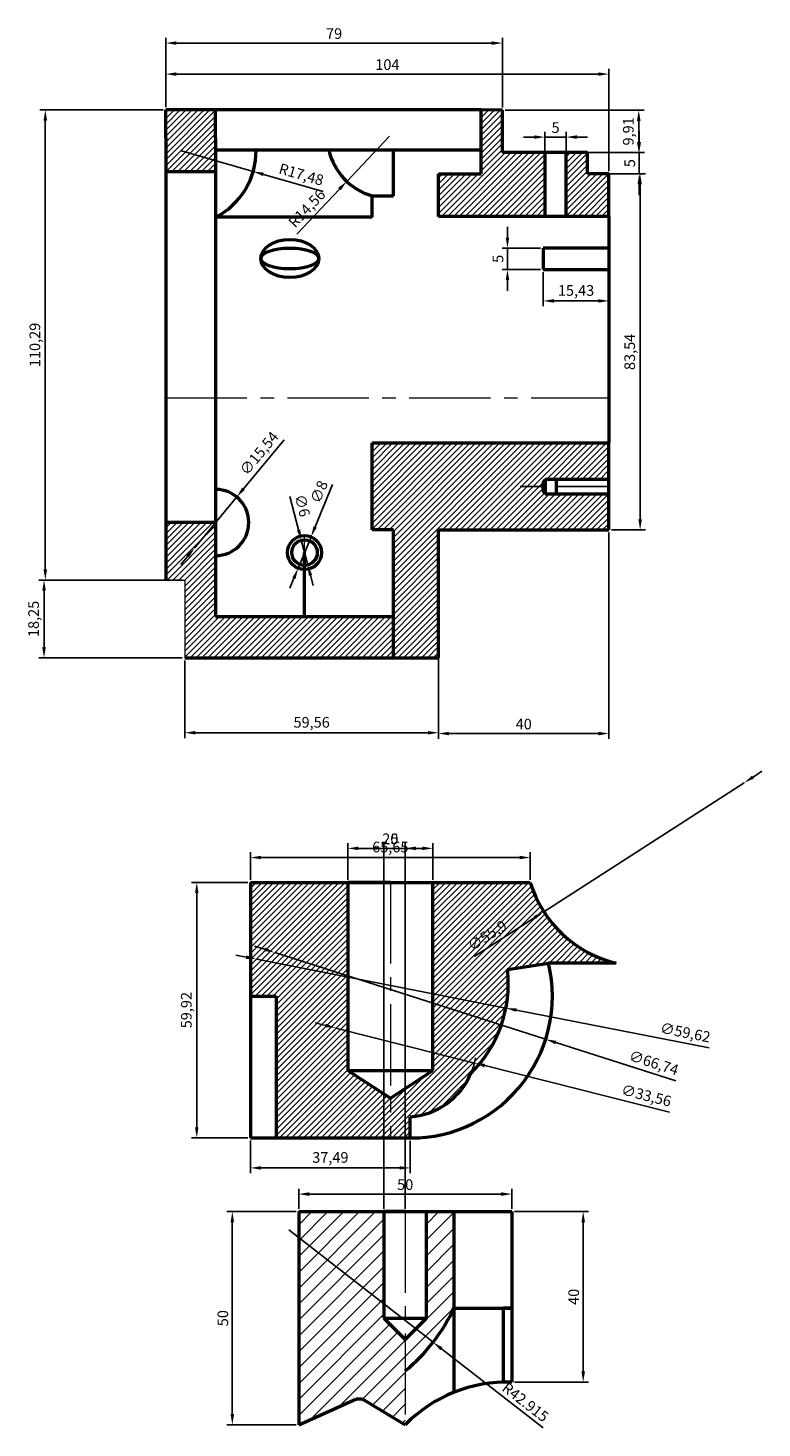
# Model space of a CAD drawing. Units: millimetres. Extents: x 1140 to 1880, y 1480 to 1815.
# Tile 2 of 3: x 1420 to 1592, y 1480 to 1809. Entities that reach past the tile are written whole.
import ezdxf

# ---------------------------------------------------------------- set-up
doc = ezdxf.new("R2010")
doc.units = ezdxf.units.MM
doc.linetypes.add('ACAD_ISO02W100', pattern=[15, 12, -3])
doc.linetypes.add('CENTER2', pattern=[28.575, 19.05, -3.175, 3.175, -3.175])
for name, color, linetype, lineweight in [('M-CNTR', 1, 'CENTER2', 18), ('M-DIMS', 2, 'Continuous', 25), ('M-HATC', 8, 'Continuous', 18), ('M-HIDN', 6, 'ACAD_ISO02W100', 25), ('M-OUTL', 7, 'Continuous', 50)]:
    doc.layers.add(name, color=color, linetype=linetype, lineweight=lineweight)
doc.styles.get("Standard").update_dxf_attribs({"font": 'arial.ttf'})
doc.dimstyles.new('ISO-25', dxfattribs={"dimtxt": 2.5, "dimasz": 2.5, "dimexe": 1.25, "dimexo": 0.625, "dimtad": 1, "dimtxsty": 'Standard', "dimcen": 2.5, "dimadec": 0, "dimazin": 0, "dimtfac": 1, "dimtmove": 0, "dimatfit": 3, "dimfxl": 1, "dimarcsym": 0})

# ---------------------------------------------------------------- blocks, each defined once
blk = doc.blocks.new('*D32')
at = {"layer": 'Defpoints', "color": 0, "transparency": 16777216}
for p in [(1451.99, 1789.45), (1423.7, 1679.16), (1451.99, 1679.16)]:
    blk.add_point(p, dxfattribs=at)
at = {"layer": 'M-DIMS', "color": 0, "lineweight": -2, "transparency": 16777216}
for p, q in [((1451.36, 1789.45), (1422.45, 1789.45)), ((1423.7, 1786.95), (1423.7, 1681.66)), ((1451.36, 1679.16), (1422.45, 1679.16))]:
    blk.add_line(p, q, dxfattribs=at)
at = {"layer": 'M-DIMS', "color": 0, "transparency": 16777216}
for points in [[(1423.28, 1786.95), (1424.12, 1786.95), (1423.7, 1789.45)], [(1423.28, 1681.66), (1424.12, 1681.66), (1423.7, 1679.16)]]:
    blk.add_solid(points, dxfattribs=at)
at = {"layer": 'M-DIMS', "color": 0, "transparency": 16777216, "insert": (1421.57, 1734.31), "char_height": 2.5, "attachment_point": 5, "rotation": 90}
blk.add_mtext('110,29', dxfattribs=at)
blk = doc.blocks.new('*D33')
at = {"layer": 'Defpoints', "color": 0, "transparency": 16777216}
for p in [(1456.43, 1679.16), (1423.4, 1660.92), (1456.43, 1660.92)]:
    blk.add_point(p, dxfattribs=at)
at = {"layer": 'M-DIMS', "color": 0, "lineweight": -2, "transparency": 16777216}
for p, q in [((1455.81, 1679.16), (1422.15, 1679.16)), ((1423.4, 1676.66), (1423.4, 1663.42)), ((1455.81, 1660.92), (1422.15, 1660.92))]:
    blk.add_line(p, q, dxfattribs=at)
at = {"layer": 'M-DIMS', "color": 0, "transparency": 16777216}
for points in [[(1422.98, 1676.66), (1423.82, 1676.66), (1423.4, 1679.16)], [(1422.98, 1663.42), (1423.82, 1663.42), (1423.4, 1660.92)]]:
    blk.add_solid(points, dxfattribs=at)
at = {"layer": 'M-DIMS', "color": 0, "transparency": 16777216, "insert": (1421.27, 1670.04), "char_height": 2.5, "attachment_point": 5, "rotation": 90}
blk.add_mtext('18,25', dxfattribs=at)
blk = doc.blocks.new('*D34')
at = {"layer": 'Defpoints', "color": 0, "transparency": 16777216}
for p in [(1530.99, 1805.12), (1451.99, 1789.45), (1530.99, 1789.36)]:
    blk.add_point(p, dxfattribs=at)
at = {"layer": 'M-DIMS', "color": 0, "lineweight": -2, "transparency": 16777216}
for p, q in [((1451.99, 1790.08), (1451.99, 1806.37)), ((1530.99, 1789.98), (1530.99, 1806.37)), ((1454.49, 1805.12), (1528.49, 1805.12))]:
    blk.add_line(p, q, dxfattribs=at)
at = {"layer": 'M-DIMS', "color": 0, "transparency": 16777216}
for points in [[(1454.49, 1805.54), (1454.49, 1804.7), (1451.99, 1805.12)], [(1528.49, 1805.54), (1528.49, 1804.7), (1530.99, 1805.12)]]:
    blk.add_solid(points, dxfattribs=at)
at = {"layer": 'M-DIMS', "color": 0, "transparency": 16777216, "insert": (1491.49, 1807.02), "char_height": 2.5, "attachment_point": 5}
blk.add_mtext('79', dxfattribs=at)
blk = doc.blocks.new('*D35')
at = {"layer": 'Defpoints', "color": 0, "transparency": 16777216}
for p in [(1530.99, 1789.36), (1530.99, 1779.45), (1562.99, 1779.45)]:
    blk.add_point(p, dxfattribs=at)
at = {"layer": 'M-DIMS', "color": 0, "lineweight": -2, "transparency": 16777216}
for p, q in [((1531.61, 1789.36), (1564.24, 1789.36)), ((1562.99, 1786.86), (1562.99, 1781.95)), ((1531.61, 1779.45), (1564.24, 1779.45))]:
    blk.add_line(p, q, dxfattribs=at)
at = {"layer": 'M-DIMS', "color": 0, "transparency": 16777216}
for points in [[(1562.57, 1786.86), (1563.41, 1786.86), (1562.99, 1789.36)], [(1562.57, 1781.95), (1563.41, 1781.95), (1562.99, 1779.45)]]:
    blk.add_solid(points, dxfattribs=at)
at = {"layer": 'M-DIMS', "color": 0, "transparency": 16777216, "insert": (1560.86, 1784.41), "char_height": 2.5, "attachment_point": 5, "rotation": 90}
blk.add_mtext('9,91', dxfattribs=at)
blk = doc.blocks.new('*D36')
at = {"layer": 'Defpoints', "color": 0, "transparency": 16777216}
for p in [(1550.99, 1779.45), (1550.99, 1774.45), (1563.11, 1774.45)]:
    blk.add_point(p, dxfattribs=at)
at = {"layer": 'M-DIMS', "color": 0, "lineweight": -2, "transparency": 16777216}
for p, q in [((1563.11, 1781.95), (1563.11, 1784.45)), ((1551.61, 1779.45), (1564.36, 1779.45)), ((1563.11, 1779.45), (1563.11, 1774.45)), ((1551.61, 1774.45), (1564.36, 1774.45)), ((1563.11, 1771.95), (1563.11, 1769.45))]:
    blk.add_line(p, q, dxfattribs=at)
at = {"layer": 'M-DIMS', "color": 0, "transparency": 16777216}
for points in [[(1562.69, 1781.95), (1563.53, 1781.95), (1563.11, 1779.45)], [(1562.69, 1771.95), (1563.53, 1771.95), (1563.11, 1774.45)]]:
    blk.add_solid(points, dxfattribs=at)
at = {"layer": 'M-DIMS', "color": 0, "transparency": 16777216, "insert": (1561.21, 1776.95), "char_height": 2.5, "attachment_point": 5, "rotation": 90}
blk.add_mtext('5', dxfattribs=at)
blk = doc.blocks.new('*D37')
at = {"layer": 'Defpoints', "color": 0, "transparency": 16777216}
for p in [(1555.99, 1774.45), (1555.99, 1690.92), (1563.31, 1690.92)]:
    blk.add_point(p, dxfattribs=at)
at = {"layer": 'M-DIMS', "color": 0, "lineweight": -2, "transparency": 16777216}
for p, q in [((1556.61, 1774.45), (1564.56, 1774.45)), ((1563.31, 1771.95), (1563.31, 1693.42)), ((1556.61, 1690.92), (1564.56, 1690.92))]:
    blk.add_line(p, q, dxfattribs=at)
at = {"layer": 'M-DIMS', "color": 0, "transparency": 16777216}
for points in [[(1562.9, 1771.95), (1563.73, 1771.95), (1563.31, 1774.45)], [(1562.9, 1693.42), (1563.73, 1693.42), (1563.31, 1690.92)]]:
    blk.add_solid(points, dxfattribs=at)
at = {"layer": 'M-DIMS', "color": 0, "transparency": 16777216, "insert": (1561.19, 1732.68), "char_height": 2.5, "attachment_point": 5, "rotation": 90}
blk.add_mtext('83,54', dxfattribs=at)
blk = doc.blocks.new('*D38')
at = {"layer": 'Defpoints', "color": 0, "transparency": 16777216}
for p in [(1515.99, 1690.92), (1555.99, 1690.92), (1555.99, 1643.15)]:
    blk.add_point(p, dxfattribs=at)
at = {"layer": 'M-DIMS', "color": 0, "lineweight": -2, "transparency": 16777216}
for p, q in [((1515.99, 1690.29), (1515.99, 1641.9)), ((1555.99, 1690.29), (1555.99, 1641.9)), ((1518.49, 1643.15), (1553.49, 1643.15))]:
    blk.add_line(p, q, dxfattribs=at)
at = {"layer": 'M-DIMS', "color": 0, "transparency": 16777216}
for points in [[(1518.49, 1643.56), (1518.49, 1642.73), (1515.99, 1643.15)], [(1553.49, 1643.56), (1553.49, 1642.73), (1555.99, 1643.15)]]:
    blk.add_solid(points, dxfattribs=at)
at = {"layer": 'M-DIMS', "color": 0, "transparency": 16777216, "insert": (1535.99, 1645.05), "char_height": 2.5, "attachment_point": 5}
blk.add_mtext('40', dxfattribs=at)
blk = doc.blocks.new('*D39')
at = {"layer": 'Defpoints', "color": 0, "transparency": 16777216}
for p in [(1456.43, 1660.92), (1515.99, 1660.92), (1515.99, 1643.34)]:
    blk.add_point(p, dxfattribs=at)
at = {"layer": 'M-DIMS', "color": 0, "lineweight": -2, "transparency": 16777216}
for p, q in [((1456.43, 1660.29), (1456.43, 1642.09)), ((1515.99, 1660.29), (1515.99, 1642.09)), ((1458.93, 1643.34), (1513.49, 1643.34))]:
    blk.add_line(p, q, dxfattribs=at)
at = {"layer": 'M-DIMS', "color": 0, "transparency": 16777216}
for points in [[(1458.93, 1643.75), (1458.93, 1642.92), (1456.43, 1643.34)], [(1513.49, 1643.75), (1513.49, 1642.92), (1515.99, 1643.34)]]:
    blk.add_solid(points, dxfattribs=at)
at = {"layer": 'M-DIMS', "color": 0, "transparency": 16777216, "insert": (1486.21, 1645.46), "char_height": 2.5, "attachment_point": 5}
blk.add_mtext('59,56', dxfattribs=at)
blk = doc.blocks.new('*D40')
at = {"layer": 'Defpoints', "color": 0, "transparency": 16777216}
for p in [(1486.07, 1689.3), (1483.02, 1681.9)]:
    blk.add_point(p, dxfattribs=at)
at = {"layer": 'M-DIMS', "color": 0, "lineweight": -2, "transparency": 16777216}
for p, q in [((1491.13, 1701.57), (1487.02, 1691.61)), ((1483.02, 1681.9), (1486.07, 1689.3)), ((1482.06, 1679.59), (1481.11, 1677.28))]:
    blk.add_line(p, q, dxfattribs=at)
at = {"layer": 'M-DIMS', "color": 0, "transparency": 16777216}
for points in [[(1486.64, 1691.77), (1487.41, 1691.45), (1486.07, 1689.3)], [(1481.68, 1679.75), (1482.45, 1679.43), (1483.02, 1681.9)]]:
    blk.add_solid(points, dxfattribs=at)
at = {"layer": 'M-DIMS', "color": 0, "transparency": 16777216, "insert": (1488.24, 1699.72), "char_height": 2.5, "attachment_point": 5, "rotation": 67.5752}
blk.add_mtext('∅8', dxfattribs=at)
blk = doc.blocks.new('*D41')
at = {"layer": 'Defpoints', "color": 0, "transparency": 16777216}
for p in [(1483.78, 1688.5), (1485.3, 1682.7)]:
    blk.add_point(p, dxfattribs=at)
at = {"layer": 'M-DIMS', "color": 0, "lineweight": -2, "transparency": 16777216}
for p, q in [((1481.1, 1698.76), (1483.15, 1690.92)), ((1485.3, 1682.7), (1483.78, 1688.5)), ((1485.94, 1680.28), (1486.57, 1677.86))]:
    blk.add_line(p, q, dxfattribs=at)
at = {"layer": 'M-DIMS', "color": 0, "transparency": 16777216}
for points in [[(1483.56, 1691.03), (1482.75, 1690.81), (1483.78, 1688.5)], [(1486.34, 1680.38), (1485.53, 1680.17), (1485.3, 1682.7)]]:
    blk.add_solid(points, dxfattribs=at)
at = {"layer": 'M-DIMS', "color": 0, "transparency": 16777216, "insert": (1483.72, 1696.55), "char_height": 2.5, "attachment_point": 5, "rotation": 284.6546}
blk.add_mtext('∅6', dxfattribs=at)
blk = doc.blocks.new('*D42')
at = {"layer": 'Defpoints', "color": 0, "transparency": 16777216}
for p in [(1468.63, 1698.64), (1458.72, 1686.67)]:
    blk.add_point(p, dxfattribs=at)
at = {"layer": 'M-DIMS', "color": 0, "lineweight": -2, "transparency": 16777216}
for p, q in [((1479.74, 1712.07), (1470.22, 1700.57)), ((1458.72, 1686.67), (1468.63, 1698.64)), ((1457.13, 1684.75), (1455.53, 1682.82))]:
    blk.add_line(p, q, dxfattribs=at)
at = {"layer": 'M-DIMS', "color": 0, "transparency": 16777216}
for points in [[(1469.9, 1700.84), (1470.54, 1700.3), (1468.63, 1698.64)], [(1456.81, 1685.01), (1457.45, 1684.48), (1458.72, 1686.67)]]:
    blk.add_solid(points, dxfattribs=at)
at = {"layer": 'M-DIMS', "color": 0, "transparency": 16777216, "insert": (1474.12, 1708.68), "char_height": 2.5, "attachment_point": 5, "rotation": 50.3902}
blk.add_mtext('∅15,54', dxfattribs=at)
blk = doc.blocks.new('*D43')
at = {"layer": 'Defpoints', "color": 0, "transparency": 16777216}
for p in [(1540.56, 1752.01), (1555.99, 1752.01), (1555.99, 1744.64)]:
    blk.add_point(p, dxfattribs=at)
at = {"layer": 'M-DIMS', "color": 0, "lineweight": -2, "transparency": 16777216}
for p, q in [((1540.56, 1751.38), (1540.56, 1743.39)), ((1555.99, 1751.38), (1555.99, 1743.39)), ((1543.06, 1744.64), (1553.49, 1744.64))]:
    blk.add_line(p, q, dxfattribs=at)
at = {"layer": 'M-DIMS', "color": 0, "transparency": 16777216}
for points in [[(1543.06, 1745.05), (1543.06, 1744.22), (1540.56, 1744.64)], [(1553.49, 1745.05), (1553.49, 1744.22), (1555.99, 1744.64)]]:
    blk.add_solid(points, dxfattribs=at)
at = {"layer": 'M-DIMS', "color": 0, "transparency": 16777216, "insert": (1548.27, 1746.76), "char_height": 2.5, "attachment_point": 5}
blk.add_mtext('15,43', dxfattribs=at)
blk = doc.blocks.new('*D44')
at = {"layer": 'Defpoints', "color": 0, "transparency": 16777216}
for p in [(1540.56, 1757.01), (1532.18, 1752.01), (1540.56, 1752.01)]:
    blk.add_point(p, dxfattribs=at)
at = {"layer": 'M-DIMS', "color": 0, "lineweight": -2, "transparency": 16777216}
for p, q in [((1532.18, 1759.51), (1532.18, 1762.01)), ((1539.93, 1757.01), (1530.93, 1757.01)), ((1532.18, 1757.01), (1532.18, 1752.01)), ((1539.93, 1752.01), (1530.93, 1752.01)), ((1532.18, 1749.51), (1532.18, 1747.01))]:
    blk.add_line(p, q, dxfattribs=at)
at = {"layer": 'M-DIMS', "color": 0, "transparency": 16777216}
for points in [[(1531.76, 1759.51), (1532.6, 1759.51), (1532.18, 1757.01)], [(1531.76, 1749.51), (1532.6, 1749.51), (1532.18, 1752.01)]]:
    blk.add_solid(points, dxfattribs=at)
at = {"layer": 'M-DIMS', "color": 0, "transparency": 16777216, "insert": (1530.28, 1754.51), "char_height": 2.5, "attachment_point": 5, "rotation": 90}
blk.add_mtext('5', dxfattribs=at)
blk = doc.blocks.new('*D45')
at = {"layer": 'Defpoints', "color": 0, "transparency": 16777216}
for p in [(1545.97, 1783.07), (1540.97, 1764.45), (1545.97, 1764.45)]:
    blk.add_point(p, dxfattribs=at)
at = {"layer": 'M-DIMS', "color": 0, "lineweight": -2, "transparency": 16777216}
for p, q in [((1540.97, 1765.08), (1540.97, 1784.32)), ((1545.97, 1765.08), (1545.97, 1784.32)), ((1538.47, 1783.07), (1535.97, 1783.07)), ((1540.97, 1783.07), (1545.97, 1783.07)), ((1548.47, 1783.07), (1550.97, 1783.07))]:
    blk.add_line(p, q, dxfattribs=at)
at = {"layer": 'M-DIMS', "color": 0, "transparency": 16777216}
for points in [[(1538.47, 1783.49), (1538.47, 1782.66), (1540.97, 1783.07)], [(1548.47, 1783.49), (1548.47, 1782.66), (1545.97, 1783.07)]]:
    blk.add_solid(points, dxfattribs=at)
at = {"layer": 'M-DIMS', "color": 0, "transparency": 16777216, "insert": (1543.47, 1784.97), "char_height": 2.5, "attachment_point": 5}
blk.add_mtext('5', dxfattribs=at)
blk = doc.blocks.new('*D46')
at = {"layer": 'Defpoints', "color": 0, "transparency": 16777216}
for p in [(1504.46, 1783.25), (1494.45, 1772.68)]:
    blk.add_point(p, dxfattribs=at)
at = {"layer": 'M-DIMS', "color": 0, "lineweight": -2, "transparency": 16777216}
for p, q in [((1504.46, 1783.25), (1494.45, 1772.68)), ((1482.71, 1760.28), (1492.73, 1770.86))]:
    blk.add_line(p, q, dxfattribs=at)
at = {"layer": 'M-DIMS', "color": 0, "transparency": 16777216}
blk.add_solid([(1492.43, 1771.15), (1493.04, 1770.58), (1494.45, 1772.68)], dxfattribs=at)
at = {"layer": 'M-DIMS', "color": 0, "transparency": 16777216, "insert": (1485.32, 1766.13), "char_height": 2.5, "attachment_point": 5, "rotation": 46.5563}
blk.add_mtext('R14,56', dxfattribs=at)
blk = doc.blocks.new('*D47')
at = {"layer": 'Defpoints', "color": 0, "transparency": 16777216}
for p in [(1455.69, 1779.81), (1472.49, 1775)]:
    blk.add_point(p, dxfattribs=at)
at = {"layer": 'M-DIMS', "color": 0, "lineweight": -2, "transparency": 16777216}
for p, q in [((1455.69, 1779.81), (1472.49, 1775)), ((1488.92, 1770.3), (1474.9, 1774.32))]:
    blk.add_line(p, q, dxfattribs=at)
at = {"layer": 'M-DIMS', "color": 0, "transparency": 16777216}
blk.add_solid([(1475.01, 1774.72), (1474.78, 1773.92), (1472.49, 1775)], dxfattribs=at)
at = {"layer": 'M-DIMS', "color": 0, "transparency": 16777216, "insert": (1483.7, 1774.01), "char_height": 2.5, "attachment_point": 5, "rotation": 344.0331}
blk.add_mtext('R17,48', dxfattribs=at)
blk = doc.blocks.new('*D48')
at = {"layer": 'Defpoints', "color": 0, "transparency": 16777216}
for p in [(1477.56, 1591.77), (1541.13, 1571.43)]:
    blk.add_point(p, dxfattribs=at)
at = {"layer": 'M-DIMS', "color": 0, "lineweight": -2, "transparency": 16777216}
for p, q in [((1475.18, 1592.53), (1472.8, 1593.3)), ((1477.56, 1591.77), (1541.13, 1571.43)), ((1571.67, 1561.65), (1543.51, 1570.67))]:
    blk.add_line(p, q, dxfattribs=at)
at = {"layer": 'M-DIMS', "color": 0, "transparency": 16777216}
for points in [[(1475.31, 1592.93), (1475.05, 1592.14), (1477.56, 1591.77)], [(1543.63, 1571.06), (1543.38, 1570.27), (1541.13, 1571.43)]]:
    blk.add_solid(points, dxfattribs=at)
at = {"layer": 'M-DIMS', "color": 0, "transparency": 16777216, "insert": (1566.43, 1565.6), "char_height": 2.5, "attachment_point": 5, "rotation": 342.2515}
blk.add_mtext('∅66,74', dxfattribs=at)
blk = doc.blocks.new('*D49')
at = {"layer": 'Defpoints', "color": 0, "transparency": 16777216}
for p in [(1473.31, 1590.21), (1531.81, 1578.75)]:
    blk.add_point(p, dxfattribs=at)
at = {"layer": 'M-DIMS', "color": 0, "lineweight": -2, "transparency": 16777216}
for p, q in [((1470.85, 1590.7), (1468.4, 1591.18)), ((1473.31, 1590.21), (1531.81, 1578.75)), ((1579.51, 1569.4), (1534.26, 1578.27))]:
    blk.add_line(p, q, dxfattribs=at)
at = {"layer": 'M-DIMS', "color": 0, "transparency": 16777216}
for points in [[(1470.93, 1591.1), (1470.77, 1590.29), (1473.31, 1590.21)], [(1534.34, 1578.67), (1534.18, 1577.86), (1531.81, 1578.75)]]:
    blk.add_solid(points, dxfattribs=at)
at = {"layer": 'M-DIMS', "color": 0, "transparency": 16777216, "insert": (1573.85, 1572.71), "char_height": 2.5, "attachment_point": 5, "rotation": 348.9096}
blk.add_mtext('∅59,62', dxfattribs=at)
blk = doc.blocks.new('*D50')
at = {"layer": 'Defpoints', "color": 0, "transparency": 16777216}
for p in [(1491.86, 1574.07), (1524.4, 1565.86)]:
    blk.add_point(p, dxfattribs=at)
at = {"layer": 'M-DIMS', "color": 0, "lineweight": -2, "transparency": 16777216}
for p, q in [((1489.44, 1574.68), (1487.02, 1575.29)), ((1491.86, 1574.07), (1524.4, 1565.86)), ((1570.18, 1554.31), (1526.83, 1565.25))]:
    blk.add_line(p, q, dxfattribs=at)
blk.add_arc((1508.13, 1569.97), 16.78, 338.7328, 350.1075, dxfattribs=at)
at = {"layer": 'M-DIMS', "color": 0, "transparency": 16777216}
for points in [[(1489.54, 1575.09), (1489.34, 1574.28), (1491.86, 1574.07)], [(1526.93, 1565.65), (1526.73, 1564.85), (1524.4, 1565.86)]]:
    blk.add_solid(points, dxfattribs=at)
at = {"layer": 'M-DIMS', "color": 0, "transparency": 16777216, "insert": (1564.69, 1557.93), "char_height": 2.5, "attachment_point": 5, "rotation": 345.8393}
blk.add_mtext('∅33,56', dxfattribs=at)
blk = doc.blocks.new('*D51')
at = {"layer": 'Defpoints', "color": 0, "transparency": 16777216}
for p in [(1587.72, 1631.59), (1540.7, 1601.36)]:
    blk.add_point(p, dxfattribs=at)
at = {"layer": 'M-DIMS', "color": 0, "lineweight": -2, "transparency": 16777216}
for p, q in [((1589.82, 1632.94), (1591.92, 1634.29)), ((1587.72, 1631.59), (1540.7, 1601.36)), ((1524.37, 1590.86), (1538.6, 1600.01))]:
    blk.add_line(p, q, dxfattribs=at)
at = {"layer": 'M-DIMS', "color": 0, "transparency": 16777216}
for points in [[(1589.6, 1633.29), (1590.05, 1632.59), (1587.72, 1631.59)], [(1538.37, 1600.36), (1538.82, 1599.66), (1540.7, 1601.36)]]:
    blk.add_solid(points, dxfattribs=at)
at = {"layer": 'M-DIMS', "color": 0, "transparency": 16777216, "insert": (1527.6, 1595.52), "char_height": 2.5, "attachment_point": 5, "rotation": 32.7355}
blk.add_mtext('∅55,9', dxfattribs=at)
blk = doc.blocks.new('*D52')
at = {"layer": 'Defpoints', "color": 0, "transparency": 16777216}
for p in [(1537.51, 1614.07), (1471.86, 1608.21), (1537.51, 1608.21)]:
    blk.add_point(p, dxfattribs=at)
at = {"layer": 'M-DIMS', "color": 0, "lineweight": -2, "transparency": 16777216}
for p, q in [((1471.86, 1608.84), (1471.86, 1615.32)), ((1474.36, 1614.07), (1535.01, 1614.07)), ((1537.51, 1608.84), (1537.51, 1615.32))]:
    blk.add_line(p, q, dxfattribs=at)
at = {"layer": 'M-DIMS', "color": 0, "transparency": 16777216}
for points in [[(1474.36, 1614.48), (1474.36, 1613.65), (1471.86, 1614.07)], [(1535.01, 1614.48), (1535.01, 1613.65), (1537.51, 1614.07)]]:
    blk.add_solid(points, dxfattribs=at)
at = {"layer": 'M-DIMS', "color": 0, "transparency": 16777216, "insert": (1504.68, 1616.2), "char_height": 2.5, "attachment_point": 5}
blk.add_mtext('65,65', dxfattribs=at)
blk = doc.blocks.new('*D53')
at = {"layer": 'Defpoints', "color": 0, "transparency": 16777216}
for p in [(1471.86, 1608.21), (1459.24, 1548.3), (1471.86, 1548.3)]:
    blk.add_point(p, dxfattribs=at)
at = {"layer": 'M-DIMS', "color": 0, "lineweight": -2, "transparency": 16777216}
for p, q in [((1471.23, 1608.21), (1457.99, 1608.21)), ((1459.24, 1605.71), (1459.24, 1550.8)), ((1471.23, 1548.3), (1457.99, 1548.3))]:
    blk.add_line(p, q, dxfattribs=at)
at = {"layer": 'M-DIMS', "color": 0, "transparency": 16777216}
for points in [[(1458.83, 1605.71), (1459.66, 1605.71), (1459.24, 1608.21)], [(1458.83, 1550.8), (1459.66, 1550.8), (1459.24, 1548.3)]]:
    blk.add_solid(points, dxfattribs=at)
at = {"layer": 'M-DIMS', "color": 0, "transparency": 16777216, "insert": (1457.12, 1578.26), "char_height": 2.5, "attachment_point": 5, "rotation": 90}
blk.add_mtext('59,92', dxfattribs=at)
blk = doc.blocks.new('*D54')
at = {"layer": 'Defpoints', "color": 0, "transparency": 16777216}
for p in [(1471.86, 1548.3), (1509.34, 1548.23), (1509.34, 1541.25)]:
    blk.add_point(p, dxfattribs=at)
at = {"layer": 'M-DIMS', "color": 0, "lineweight": -2, "transparency": 16777216}
for p, q in [((1471.86, 1547.67), (1471.86, 1540)), ((1509.34, 1547.6), (1509.34, 1540)), ((1474.36, 1541.25), (1506.84, 1541.25))]:
    blk.add_line(p, q, dxfattribs=at)
at = {"layer": 'M-DIMS', "color": 0, "transparency": 16777216}
for points in [[(1474.36, 1541.67), (1474.36, 1540.84), (1471.86, 1541.25)], [(1506.84, 1541.67), (1506.84, 1540.84), (1509.34, 1541.25)]]:
    blk.add_solid(points, dxfattribs=at)
at = {"layer": 'M-DIMS', "color": 0, "transparency": 16777216, "insert": (1490.6, 1543.38), "char_height": 2.5, "attachment_point": 5}
blk.add_mtext('37,49', dxfattribs=at)
blk = doc.blocks.new('*D55')
at = {"layer": 'Defpoints', "color": 0, "transparency": 16777216}
for p in [(1533.17, 1535.11), (1483.17, 1531), (1533.17, 1531)]:
    blk.add_point(p, dxfattribs=at)
at = {"layer": 'M-DIMS', "color": 0, "lineweight": -2, "transparency": 16777216}
for p, q in [((1483.17, 1531.63), (1483.17, 1536.36)), ((1485.67, 1535.11), (1530.67, 1535.11)), ((1533.17, 1531.63), (1533.17, 1536.36))]:
    blk.add_line(p, q, dxfattribs=at)
at = {"layer": 'M-DIMS', "color": 0, "transparency": 16777216}
for points in [[(1485.67, 1535.53), (1485.67, 1534.69), (1483.17, 1535.11)], [(1530.67, 1535.53), (1530.67, 1534.69), (1533.17, 1535.11)]]:
    blk.add_solid(points, dxfattribs=at)
at = {"layer": 'M-DIMS', "color": 0, "transparency": 16777216, "insert": (1508.17, 1537.01), "char_height": 2.5, "attachment_point": 5}
blk.add_mtext('50', dxfattribs=at)
blk = doc.blocks.new('*D56')
at = {"layer": 'Defpoints', "color": 0, "transparency": 16777216}
for p in [(1483.17, 1531), (1467.59, 1481), (1483.17, 1481)]:
    blk.add_point(p, dxfattribs=at)
at = {"layer": 'M-DIMS', "color": 0, "lineweight": -2, "transparency": 16777216}
for p, q in [((1482.55, 1531), (1466.34, 1531)), ((1467.59, 1528.5), (1467.59, 1483.5)), ((1482.55, 1481), (1466.34, 1481))]:
    blk.add_line(p, q, dxfattribs=at)
at = {"layer": 'M-DIMS', "color": 0, "transparency": 16777216}
for points in [[(1467.18, 1528.5), (1468.01, 1528.5), (1467.59, 1531)], [(1467.18, 1483.5), (1468.01, 1483.5), (1467.59, 1481)]]:
    blk.add_solid(points, dxfattribs=at)
at = {"layer": 'M-DIMS', "color": 0, "transparency": 16777216, "insert": (1465.69, 1506), "char_height": 2.5, "attachment_point": 5, "rotation": 90}
blk.add_mtext('50', dxfattribs=at)
blk = doc.blocks.new('*D57')
at = {"layer": 'Defpoints', "color": 0, "transparency": 16777216}
for p in [(1533.17, 1531), (1533.17, 1491), (1549.95, 1491)]:
    blk.add_point(p, dxfattribs=at)
at = {"layer": 'M-DIMS', "color": 0, "lineweight": -2, "transparency": 16777216}
for p, q in [((1533.8, 1531), (1551.2, 1531)), ((1549.95, 1528.5), (1549.95, 1493.5)), ((1533.8, 1491), (1551.2, 1491))]:
    blk.add_line(p, q, dxfattribs=at)
at = {"layer": 'M-DIMS', "color": 0, "transparency": 16777216}
for points in [[(1549.54, 1528.5), (1550.37, 1528.5), (1549.95, 1531)], [(1549.54, 1493.5), (1550.37, 1493.5), (1549.95, 1491)]]:
    blk.add_solid(points, dxfattribs=at)
at = {"layer": 'M-DIMS', "color": 0, "transparency": 16777216, "insert": (1548.05, 1511), "char_height": 2.5, "attachment_point": 5, "rotation": 90}
blk.add_mtext('40', dxfattribs=at)
blk = doc.blocks.new('*D86')
at = {"layer": 'Defpoints', "color": 0, "transparency": 16777216}
for p in [(1555.99, 1797.85), (1451.99, 1789.45), (1555.99, 1774.45)]:
    blk.add_point(p, dxfattribs=at)
at = {"layer": 'M-DIMS', "color": 0, "lineweight": -2, "transparency": 16777216}
for p, q in [((1451.99, 1790.08), (1451.99, 1799.1)), ((1454.49, 1797.85), (1553.49, 1797.85)), ((1555.99, 1775.08), (1555.99, 1799.1))]:
    blk.add_line(p, q, dxfattribs=at)
at = {"layer": 'M-DIMS', "color": 0, "transparency": 16777216}
for points in [[(1454.49, 1798.27), (1454.49, 1797.44), (1451.99, 1797.85)], [(1553.49, 1798.27), (1553.49, 1797.44), (1555.99, 1797.85)]]:
    blk.add_solid(points, dxfattribs=at)
at = {"layer": 'M-DIMS', "color": 0, "transparency": 16777216, "insert": (1503.99, 1799.75), "char_height": 2.5, "attachment_point": 5}
blk.add_mtext('104', dxfattribs=at)
blk = doc.blocks.new('*D88')
at = {"layer": 'Defpoints', "color": 0, "transparency": 16777216}
for p in [(1514.68, 1616.21), (1494.68, 1608.21), (1514.68, 1608.21)]:
    blk.add_point(p, dxfattribs=at)
at = {"layer": 'M-DIMS', "color": 0, "lineweight": -2, "transparency": 16777216}
for p, q in [((1494.68, 1608.84), (1494.68, 1617.46)), ((1497.18, 1616.21), (1512.18, 1616.21)), ((1514.68, 1608.84), (1514.68, 1617.46))]:
    blk.add_line(p, q, dxfattribs=at)
at = {"layer": 'M-DIMS', "color": 0, "transparency": 16777216}
for points in [[(1497.18, 1616.63), (1497.18, 1615.8), (1494.68, 1616.21)], [(1512.18, 1616.63), (1512.18, 1615.8), (1514.68, 1616.21)]]:
    blk.add_solid(points, dxfattribs=at)
at = {"layer": 'M-DIMS', "color": 0, "transparency": 16777216, "insert": (1504.68, 1618.12), "char_height": 2.5, "attachment_point": 5}
blk.add_mtext('20', dxfattribs=at)
blk = doc.blocks.new('*D89')
at = {"layer": 'Defpoints', "color": 0, "transparency": 16777216}
for p in [(1508.17, 1616.21), (1503.17, 1531), (1508.17, 1531)]:
    blk.add_point(p, dxfattribs=at)
at = {"layer": 'M-DIMS', "color": 0, "lineweight": -2, "transparency": 16777216}
for p, q in [((1500.67, 1616.21), (1498.17, 1616.21)), ((1503.17, 1531.63), (1503.17, 1617.46)), ((1503.17, 1616.21), (1508.17, 1616.21)), ((1508.17, 1531.63), (1508.17, 1617.46)), ((1510.67, 1616.21), (1513.17, 1616.21))]:
    blk.add_line(p, q, dxfattribs=at)
at = {"layer": 'M-DIMS', "color": 0, "transparency": 16777216}
for points in [[(1500.67, 1616.63), (1500.67, 1615.8), (1503.17, 1616.21)], [(1510.67, 1616.63), (1510.67, 1615.8), (1508.17, 1616.21)]]:
    blk.add_solid(points, dxfattribs=at)
at = {"layer": 'M-DIMS', "color": 0, "transparency": 16777216, "insert": (1505.67, 1618.11), "char_height": 2.5, "attachment_point": 5}
blk.add_mtext('5', dxfattribs=at)
blk = doc.blocks.new('*D103')
at = {"layer": 'Defpoints', "color": 0, "transparency": 16777216}
for p in [(1480.82, 1526.69), (1514.7, 1500.35)]:
    blk.add_point(p, dxfattribs=at)
at = {"layer": 'M-DIMS', "color": 0, "lineweight": -2, "transparency": 16777216}
for p, q in [((1480.82, 1526.69), (1514.7, 1500.35)), ((1540.57, 1480.24), (1516.68, 1498.82))]:
    blk.add_line(p, q, dxfattribs=at)
at = {"layer": 'M-DIMS', "color": 0, "transparency": 16777216}
blk.add_solid([(1516.93, 1499.15), (1516.42, 1498.49), (1514.7, 1500.35)], dxfattribs=at)
at = {"layer": 'M-DIMS', "color": 0, "transparency": 16777216, "insert": (1536.2, 1486.05), "char_height": 2.5, "attachment_point": 5, "rotation": 322.1323}
blk.add_mtext('R42.915', dxfattribs=at)

msp = doc.modelspace()

# ---------------------------------------------------------------- hatches: boundary and pattern name
at = {"layer": 'M-HATC'}
h = msp.add_hatch(dxfattribs=at)
h.set_pattern_fill('ANSI31', color=256, scale=0.31)
h.paths.add_polyline_path([(1463.676, 1782.9151), (1463.676, 1789.4523), (1451.9882, 1789.4523), (1451.9882, 1782.9151), (1451.9882, 1774.9702), (1463.676, 1774.9702)])
h.paths.add_polyline_path([(1463.676, 1692.6575), (1451.9882, 1692.6575), (1451.9882, 1679.1615), (1456.4314, 1679.1615), (1456.4314, 1660.9151), (1505.4119, 1660.9151), (1505.4119, 1670.5987), (1463.676, 1670.5987)])
h.paths.add_polyline_path([(1555.9882, 1699.3651), (1540.9882, 1699.3651, -0.34029733), (1540.9882, 1702.7664), (1555.9882, 1702.7664), (1555.9882, 1711.3072), (1500.4119, 1711.3072), (1500.4119, 1690.9151), (1505.4119, 1690.9151), (1505.4119, 1660.9151), (1515.9882, 1660.9151), (1515.9882, 1690.9151), (1555.9882, 1690.9151)])
h.paths.add_polyline_path([(1540.966, 1779.4523), (1530.9882, 1779.4523), (1530.9882, 1789.3579), (1525.9882, 1789.4523), (1525.9882, 1774.4523), (1515.9882, 1774.4523), (1515.9882, 1764.4523), (1540.966, 1764.4523)])
h.paths.add_polyline_path([(1555.9882, 1774.4523), (1550.9882, 1774.4523), (1550.9882, 1779.4523), (1545.966, 1779.4523), (1545.966, 1764.4523), (1555.9882, 1764.4523)])
h = msp.add_hatch(dxfattribs=at)
h.set_pattern_fill('ANSI31', color=256, scale=0.31)
h.paths.add_polyline_path([(1494.6832, 1608.2147), (1471.8582, 1608.2147), (1471.8582, 1581.5175), (1477.8672, 1581.5175), (1477.8672, 1548.2983), (1504.6832, 1548.2983), (1504.6832, 1557.5846), (1494.6832, 1564.0867)])
h.paths.add_polyline_path([(1537.5082, 1608.2147), (1514.6832, 1608.2147), (1514.6832, 1564.0867), (1504.6832, 1557.5846), (1504.6832, 1548.2983), (1509.3434, 1548.2983), (1509.3434, 1553.23, 0.27949915), (1523.5327, 1563.3016, 0.22911344), (1532.1832, 1587.7724), (1541.8142, 1589.2938), (1557.7082, 1589.2938, -0.26494748)])
h = msp.add_hatch(dxfattribs=at)
h.set_pattern_fill('ANSI31', color=256, scale=0.83)
h.paths.add_polyline_path([(1503.1744, 1506.003), (1503.1744, 1531.003), (1483.1744, 1531.003), (1483.1744, 1481.003), (1496.0715, 1486.7547, -0.24431376), (1498.8332, 1486.5895), (1508.1744, 1481.003), (1508.1744, 1500.9961)])
h.paths.add_polyline_path([(1519.6134, 1531.003), (1513.1744, 1531.003), (1513.1744, 1506.003), (1508.1744, 1500.9961), (1508.1744, 1493.6235, 0.10986875), (1519.6134, 1508.3345)])

# ---------------------------------------------------------------- linework, layer by layer
at = {"layer": 'M-CNTR'}
for p, q in [((1451.9882, 1721.9151), (1555.9882, 1721.9151)), ((1484.5439, 1670.5987), (1484.5439, 1689.5987)), ((1451.9882, 1679.1615), (1456.4314, 1679.1615)), ((1456.4314, 1679.1615), (1456.4314, 1660.9151)), ((1484.5439, 1670.5987), (1484.5439, 1670.5987)), ((1504.6832, 1608.2147), (1504.6832, 1548.2983)), ((1508.1744, 1531.003), (1508.1744, 1481.003))]:
    msp.add_line(p, q, dxfattribs=at)
at = {"layer": 'M-HIDN'}
msp.add_line((1555.9882, 1701.0651), (1535.1952, 1701.0651), dxfattribs=at)
at = {"layer": 'M-OUTL'}
for p, q in [((1525.9882, 1789.4523), (1451.9882, 1789.4523)), ((1451.9882, 1782.9151), (1451.9882, 1789.4523)), ((1463.676, 1782.9151), (1463.676, 1789.4523)), ((1525.9882, 1774.4523), (1525.9882, 1789.4523)), ((1530.9882, 1789.3579), (1525.9882, 1789.4523)), ((1530.9882, 1779.4523), (1530.9882, 1789.3579)), ((1451.9882, 1782.9151), (1451.9882, 1679.1615)), ((1463.676, 1782.9151), (1463.676, 1670.5987)), ((1525.9882, 1780.0214), (1463.676, 1780.0214)), ((1505.4119, 1769.2662), (1505.4119, 1780.0214)), ((1550.9882, 1779.4523), (1530.9882, 1779.4523)), ((1540.966, 1779.4523), (1540.966, 1764.4523)), ((1545.966, 1764.4523), (1545.966, 1779.4523)), ((1550.9882, 1774.4523), (1550.9882, 1779.4523)), ((1451.9882, 1774.9702), (1463.676, 1774.9702)), ((1515.9882, 1764.4523), (1515.9882, 1774.4523)), ((1515.9882, 1774.4523), (1525.9882, 1774.4523)), ((1555.9882, 1774.4523), (1550.9882, 1774.4523)), ((1555.9882, 1764.4523), (1555.9882, 1774.4523)), ((1500.4119, 1764.2662), (1500.4119, 1769.2662)), ((1500.4119, 1769.2662), (1505.4119, 1769.2662)), ((1500.4119, 1764.2662), (1463.676, 1764.2662)), ((1555.9882, 1764.4523), (1515.9882, 1764.4523)), ((1555.9882, 1764.4523), (1555.9882, 1711.3072)), ((1555.9882, 1757.0066), (1540.5554, 1757.0066)), ((1540.5554, 1757.0066), (1540.5554, 1752.0066)), ((1540.5554, 1752.0066), (1555.9882, 1752.0066)), ((1500.4119, 1690.9151), (1500.4119, 1711.3072)), ((1500.4119, 1711.3072), (1555.9882, 1711.3072)), ((1555.9882, 1690.9151), (1555.9882, 1711.3072)), ((1555.9882, 1702.7664), (1540.9882, 1702.7664)), ((1540.9882, 1702.7664), (1540.9882, 1701.0651)), ((1543.5742, 1702.7664), (1543.5742, 1699.3651)), ((1540.9882, 1701.0651), (1540.9882, 1699.3651)), ((1540.9882, 1699.3651), (1555.9882, 1699.3651)), ((1555.9882, 1690.9151), (1555.9882, 1701.0651)), ((1463.676, 1692.6575), (1451.9882, 1692.6575)), ((1505.4119, 1690.9151), (1500.4119, 1690.9151)), ((1505.4119, 1660.9151), (1505.4119, 1690.9151)), ((1515.9882, 1660.9151), (1515.9882, 1690.9151)), ((1515.9882, 1690.9151), (1555.9882, 1690.9151)), ((1484.5439, 1670.5987), (1484.5439, 1685.5987)), ((1463.676, 1670.5987), (1505.4119, 1670.5987)), ((1484.5439, 1670.5987), (1484.5439, 1670.5987)), ((1456.4314, 1660.9151), (1515.9882, 1660.9151)), ((1471.8582, 1608.2147), (1471.8582, 1548.2983)), ((1471.8582, 1608.2147), (1537.5082, 1608.2147)), ((1504.6832, 1608.2147), (1494.6832, 1608.2147)), ((1494.6832, 1608.2147), (1494.6832, 1564.0867)), ((1504.6832, 1608.2147), (1499.6832, 1608.2147)), ((1514.6832, 1564.0867), (1514.6832, 1608.2147)), ((1532.1832, 1587.7724), (1541.8142, 1589.2938)), ((1557.7082, 1589.2938), (1541.8142, 1589.2938)), ((1471.8582, 1581.5175), (1477.8672, 1581.5175)), ((1477.8672, 1581.5175), (1477.8672, 1548.2983)), ((1494.6832, 1564.0867), (1514.6832, 1564.0867)), ((1494.6832, 1564.0867), (1504.6832, 1557.5846)), ((1504.6832, 1557.5846), (1514.6832, 1564.0867)), ((1509.3434, 1548.23), (1509.3434, 1553.23)), ((1471.8582, 1548.2983), (1511.4787, 1548.2983)), ((1483.1744, 1531.003), (1533.1744, 1531.003)), ((1483.1744, 1531.003), (1483.1744, 1481.003)), ((1508.1744, 1531.003), (1503.1744, 1531.003)), ((1503.1744, 1531.003), (1503.1744, 1506.003)), ((1513.1744, 1506.003), (1513.1744, 1531.003)), ((1519.6134, 1531.003), (1519.6134, 1488.6115)), ((1533.1744, 1531.003), (1533.1744, 1491.003)), ((1519.6134, 1508.3345), (1533.1744, 1508.3345)), ((1533.1744, 1508.3345), (1531.1744, 1508.3345)), ((1531.1744, 1508.3345), (1531.1744, 1491.0072)), ((1503.1744, 1506.003), (1513.1744, 1506.003)), ((1503.1744, 1506.003), (1508.1744, 1500.9961)), ((1508.1744, 1500.9961), (1513.1744, 1506.003)), ((1483.1744, 1481.003), (1496.0715, 1486.7547)), ((1498.8332, 1486.5895), (1508.1744, 1481.003))]:
    msp.add_line(p, q, dxfattribs=at)
for radius in [4, 3]:
    msp.add_circle((1484.5439, 1685.5987), radius, dxfattribs=at)
for centre, radius, start, end in [((1455.6927, 1779.8116), 17.4755, 297.182391, 0.687755), ((1504.4643, 1783.249), 14.5582, 192.809194, 253.837902), ((1543.1976, 1701.0657), 2.7881, 142.413396, 217.586604), ((1463.676, 1692.6575), 7.7705, 270, 90), ((1564.2085, 1616.4766), 27.9493, 197.193749, 256.551411), ((1509.3434, 1581.5998), 33.3699, 266.331325, 13.330332), ((1502.558, 1584.4806), 29.8075, 314.722482, 6.340526), ((1508.1332, 1569.966), 16.7798, 274.136152, 336.598683), ((1480.8242, 1526.6935), 42.9146, 309.592183, 334.671657), ((1532.1037, 1457.4299), 33.5902, 88.17325, 135.429569), ((1497.2934, 1484.0148), 3, 59.118656, 114.035466)]:
    msp.add_arc(centre, radius, start, end, dxfattribs=at)
for major_axis, ratio in [((-6.8203, 0), 0.6550601), ((6.8203, 0), 0.36000046)]:
    msp.add_ellipse((1481.09, 1754.5939), major_axis=major_axis, ratio=ratio, dxfattribs=at)

# ---------------------------------------------------------------- dimensions: what is measured, and where the dimension line sits
at = {"layer": 'M-DIMS'}
for base, p1, p2, override, picture, middle in [((1530.9882, 1805.1199), (1451.9882, 1789.4523), (1530.9882, 1789.3579), {"dimclrd": 0, "dimclre": 0, "dimclrt": 0}, '*D34', (1491.4882, 1807.0213)), ((1555.9882, 1797.8523), (1451.9882, 1789.4523), (1555.9882, 1774.4523), {"dimdec": 0, "dimlfac": 1, "dimrnd": 0, "dimzin": 0, "dimdsep": 46, "dimlunit": 2}, '*D86', (1503.9882, 1799.7537)), ((1545.966, 1783.0737), (1540.966, 1764.4523), (1545.966, 1764.4523), {"dimclrd": 0, "dimclre": 0, "dimclrt": 0}, '*D45', (1543.466, 1784.9701)), ((1555.9882, 1744.6356), (1540.5554, 1752.0066), (1555.9882, 1752.0066), {"dimclrd": 0, "dimclre": 0, "dimclrt": 0}, '*D43', (1548.2718, 1746.763)), ((1555.9882, 1643.1459), (1515.9882, 1690.9151), (1555.9882, 1690.9151), {"dimclrd": 0, "dimclre": 0, "dimclrt": 0}, '*D38', (1535.9882, 1645.0473)), ((1515.9882, 1643.3353), (1456.4314, 1660.9151), (1515.9882, 1660.9151), {"dimclrd": 0, "dimclre": 0, "dimclrt": 0}, '*D39', (1486.2098, 1645.4627)), ((1514.6832, 1616.2147), (1494.6832, 1608.2147), (1514.6832, 1608.2147), {"dimdec": 0, "dimlfac": 1, "dimrnd": 0, "dimzin": 0, "dimdsep": 46, "dimlunit": 2}, '*D88', (1504.6832, 1618.1161)), ((1508.1744, 1616.2147), (1503.1744, 1531.003), (1508.1744, 1531.003), {"dimdec": 0, "dimlfac": 1, "dimrnd": 0, "dimzin": 0, "dimdsep": 46, "dimlunit": 2}, '*D89', (1505.6744, 1618.111)), ((1537.5082, 1614.0679), (1471.8582, 1608.2147), (1537.5082, 1608.2147), {"dimclrd": 0, "dimclre": 0, "dimclrt": 0}, '*D52', (1504.6832, 1616.1953)), ((1509.3434, 1541.2531), (1471.8582, 1548.2983), (1509.3434, 1548.23), {"dimclrd": 0, "dimclre": 0, "dimclrt": 0}, '*D54', (1490.6008, 1543.3805)), ((1533.1744, 1535.1107), (1483.1744, 1531.003), (1533.1744, 1531.003), {"dimclrd": 0, "dimclre": 0, "dimclrt": 0}, '*D55', (1508.1744, 1537.0122))]:
    dim = msp.add_linear_dim(base=base, p1=p1, p2=p2, dimstyle='ISO-25', override=override, dxfattribs=at)
    dim.commit()
    dim.dimension.update_dxf_attribs({"geometry": picture, "text_midpoint": middle})
for base, p1, p2, picture, middle in [((1423.7002, 1679.1615), (1451.9882, 1789.4523), (1451.9882, 1679.1615), '*D32', (1421.5728, 1734.3069)), ((1562.9916, 1779.4523), (1530.9882, 1789.3579), (1530.9882, 1779.4523), '*D35', (1560.8643, 1784.4051)), ((1563.1102, 1774.4523), (1550.9882, 1779.4523), (1550.9882, 1774.4523), '*D36', (1561.2139, 1776.9523)), ((1563.3147, 1690.9151), (1555.9882, 1774.4523), (1555.9882, 1690.9151), '*D37', (1561.1873, 1732.6837)), ((1532.1803, 1752.0066), (1540.5554, 1757.0066), (1540.5554, 1752.0066), '*D44', (1530.284, 1754.5066)), ((1423.3991, 1660.9151), (1456.4314, 1679.1615), (1456.4314, 1660.9151), '*D33', (1421.2717, 1670.0383)), ((1459.2444, 1548.2983), (1471.8582, 1608.2147), (1471.8582, 1548.2983), '*D53', (1457.1171, 1578.2565)), ((1467.5924, 1481.003), (1483.1744, 1531.003), (1483.1744, 1481.003), '*D56', (1465.691, 1506.003)), ((1549.9531, 1491.003), (1533.1744, 1531.003), (1533.1744, 1491.003), '*D57', (1548.0516, 1511.003))]:
    dim = msp.add_linear_dim(base=base, p1=p1, p2=p2, angle=90, dimstyle='ISO-25', override={"dimclrd": 0, "dimclre": 0, "dimclrt": 0}, dxfattribs=at)
    dim.commit()
    dim.dimension.update_dxf_attribs({"geometry": picture, "text_midpoint": middle})
for center, mpoint, picture, middle in [((1504.4643, 1783.249), (1494.4534, 1772.679), '*D46', (1485.3183, 1766.1273)), ((1455.6927, 1779.8116), (1472.494, 1775.0044), '*D47', (1483.6952, 1774.0123))]:
    dim = msp.add_radius_dim(center=center, mpoint=mpoint, dimstyle='ISO-25', override={"dimclrd": 0, "dimclre": 0, "dimclrt": 0}, dxfattribs=at)
    dim.commit()
    dim.dimension.update_dxf_attribs({"geometry": picture, "text_midpoint": middle})
for p1, p2, picture, middle in [((1458.7219, 1686.6711), (1468.6301, 1698.6439), '*D42', (1475.7877, 1707.2929)), ((1483.018, 1681.9012), (1486.0698, 1689.2963), '*D40', (1490.0631, 1698.9729)), ((1587.7187, 1631.5905), (1540.6982, 1601.3627), '*D51', (1528.7709, 1593.6952)), ((1477.5619, 1591.7723), (1541.125, 1571.4274), '*D48', (1565.77, 1563.5392)), ((1473.30707, 1590.21425), (1531.80883, 1578.74688), '*D49', (1573.43733, 1570.58696)), ((1491.8633, 1574.0711), (1524.4031, 1565.861), '*D50', (1564.1614, 1555.8295))]:
    dim = msp.add_diameter_dim_2p(p1=p1, p2=p2, dimstyle='ISO-25', override={"dimclrd": 0, "dimclre": 0, "dimclrt": 0}, dxfattribs=at)
    dim.commit()
    dim.dimension.update_dxf_attribs({"geometry": picture, "text_midpoint": middle, "dimtype": 163})
dim = msp.add_diameter_dim_2p(p1=(1485.3029, 1682.6963), p2=(1483.785, 1688.5011), dimstyle='ISO-25', override={"dimclrd": 0, "dimclre": 0, "dimclrt": 0}, dxfattribs=at)
dim.commit()
dim.dimension.update_dxf_attribs({"geometry": '*D41', "text_midpoint": (1483.7179, 1696.5496)})
dim = msp.add_radius_dim(center=(1480.8242, 1526.6935), mpoint=(1514.7022, 1500.3508), dimstyle='ISO-25', override={"dimdec": 3, "dimlfac": 1, "dimrnd": 0, "dimzin": 0, "dimdsep": 46, "dimlunit": 2}, dxfattribs=at)
dim.commit()
dim.dimension.update_dxf_attribs({"geometry": '*D103', "text_midpoint": (1535.0291, 1484.5452), "dimtype": 164})

doc.saveas('drawing.dxf')
